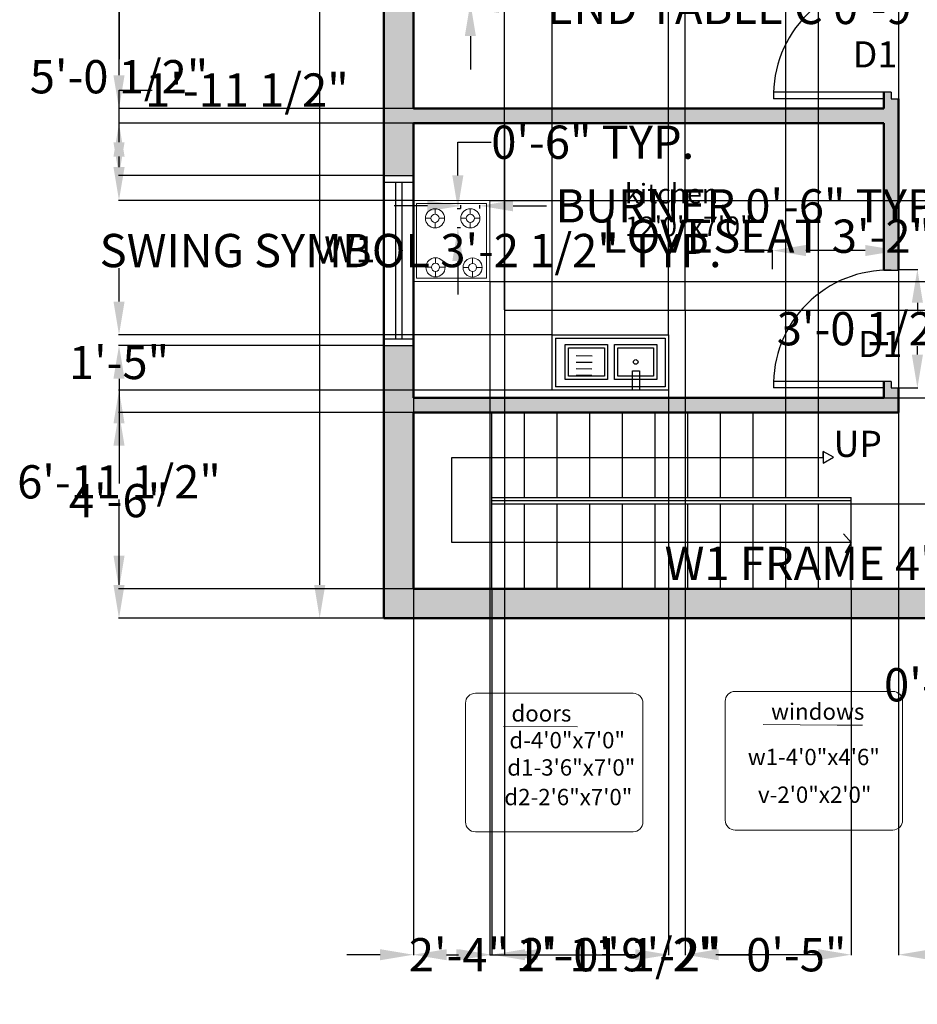
# Model space of a CAD drawing. Units: inches. Extents: x 2391 to 2964, y 130 to 798.
# Tile 1 of 4: x 2391 to 2666, y 130 to 431. Entities that reach past the tile are written whole.
import ezdxf

# ---------------------------------------------------------------- set-up
doc = ezdxf.new("R2010")
doc.units = ezdxf.units.IN
doc.header["$MEASUREMENT"] = 0
for name, color, linetype, lineweight in [('A-ANNO-DIMS', 2, 'Continuous', 18), ('A-ANNO-LEGN', 7, 'Continuous', 18), ('A-ANNO-TEXT', 7, 'Continuous', 18), ('A-AREA-IDEN', 7, 'Continuous', 25), ('A-DOOR', 3, 'Continuous', 25), ('A-EQPM', 9, 'Continuous', 18), ('A-FLOR-CASE', 8, 'Continuous', 25), ('A-FLOR-FIXT', 9, 'Continuous', 25), ('A-FLOR-STRS', 7, 'Continuous', 30), ('A-GLAZ', 4, 'Continuous', 25), ('A-WALL', 7, 'Continuous', 50)]:
    doc.layers.add(name, color=color, linetype=linetype, lineweight=lineweight)
doc.layers.add('A-WALL-PATT', color=11, linetype='Continuous', lineweight=13, true_color=0xf27172)
doc.styles.get("Standard").update_dxf_attribs({"font": 'arial.ttf'})
doc.dimstyles.get("Standard").update_dxf_attribs({"dimtxt": 10.18, "dimasz": 10.18, "dimexe": 0.18, "dimexo": 0.0625, "dimgap": 0.09, "dimtad": 0, "dimtih": 1, "dimtoh": 1, "dimdec": 0, "dimzin": 0, "dimdsep": 46, "dimlunit": 3, "dimtxsty": 'Standard', "dimcen": 0.09, "dimadec": 0, "dimazin": 0, "dimtfac": 1, "dimtdec": 0, "dimtofl": 0, "dimtmove": 0, "dimatfit": 3, "dimfxl": 1, "dimtolj": 1, "dimtzin": 0, "dimarcsym": 0})

# ---------------------------------------------------------------- blocks, each defined once
blk = doc.blocks.new('*D4')
at = {"layer": 'A-ANNO-DIMS', "color": 0, "lineweight": -2, "transparency": 16777216}
for p, q in [((2502.34, 752.24), (2482.55, 752.24)), ((2482.73, 742.06), (2482.73, 505.44)), ((2482.73, 258.42), (2482.73, 495.03)), ((2502.34, 248.24), (2482.55, 248.24))]:
    blk.add_line(p, q, dxfattribs=at)
at = {"layer": 'A-ANNO-DIMS', "color": 0, "transparency": 16777216}
for points in [[(2481.03, 742.06), (2484.43, 742.06), (2482.73, 752.24)], [(2481.03, 258.42), (2484.43, 258.42), (2482.73, 248.24)]]:
    blk.add_solid(points, dxfattribs=at)
at = {"layer": 'Defpoints', "color": 0, "transparency": 16777216}
for p in [(2502.4, 752.24), (2482.73, 248.24), (2502.4, 248.24)]:
    blk.add_point(p, dxfattribs=at)
at = {"layer": 'A-ANNO-DIMS', "color": 0, "transparency": 16777216, "insert": (2482.73, 500.24), "char_height": 10.18, "attachment_point": 5}
blk.add_mtext("\\A1;42'", dxfattribs=at)
blk = doc.blocks.new('WIN-W1-48')
for p, q in [((0, 0), (0, 9)), ((2, 0), (2, 9)), ((50, 0), (50, 9)), ((52, 0), (52, 9)), ((2, 5.5), (50, 5.5)), ((2, 3.5), (50, 3.5))]:
    blk.add_line(p, q)
blk = doc.blocks.new('DOOR-SWING-36')
for p, q in [((0, 4.5), (0, 38.25)), ((2, 2.25), (2, 38.25)), ((36, 4.5), (36, 0)), ((0, 2.25), (0, 0)), ((2, 2.25), (0, 2.25))]:
    blk.add_line(p, q)
blk.add_arc((1, 3.25), 35.01, 358.3634, 91.6366)
blk = doc.blocks.new('HOB-BURNER')
for p, q in [((2.93, 4.17), (2.93, 5.86)), ((1.69, 2.93), (0, 2.93)), ((2.93, 1.69), (2.93, 0)), ((4.17, 2.93), (5.86, 2.93))]:
    blk.add_line(p, q)
for radius in [2.93, 1.24]:
    blk.add_circle((2.93, 2.93), radius)
blk = doc.blocks.new('LEGEND-FRAME')
blk.add_line((11.62, 32.27), (34.31, 32.13))
blk.add_lwpolyline([(0, 39.41, -0.414214), (3, 42.41), (51.31, 42.41, -0.414214), (54.31, 39.41), (54.31, 3, -0.414214), (51.31, 0), (3, 0, -0.414214), (0, 3)], format="xyb", close=True)
blk = doc.blocks.new('*D15')
at = {"layer": 'A-ANNO-DIMS', "color": 0, "lineweight": -2, "transparency": 16777216}
for p, q in [((2735.63, 257.3), (2735.63, 265.22)), ((2787.63, 257.3), (2787.63, 265.22)), ((2735.63, 265.04), (2725.45, 265.04)), ((2777.45, 265.04), (2745.81, 265.04))]:
    blk.add_line(p, q, dxfattribs=at)
at = {"layer": 'A-ANNO-DIMS', "color": 0, "transparency": 16777216}
for points in [[(2745.81, 266.73), (2745.81, 263.34), (2735.63, 265.04)], [(2777.45, 266.73), (2777.45, 263.34), (2787.63, 265.04)]]:
    blk.add_solid(points, dxfattribs=at)
at = {"layer": 'Defpoints', "color": 0, "transparency": 16777216}
for p in [(2735.63, 265.04), (2735.63, 257.24), (2787.63, 257.24)]:
    blk.add_point(p, dxfattribs=at)
at = {"layer": 'A-ANNO-DIMS', "color": 0, "transparency": 16777216, "insert": (2654.62, 265.04), "char_height": 10.18, "attachment_point": 5}
blk.add_mtext('\\A1;W1 FRAME 4\'-4" TYP.', dxfattribs=at)
blk = doc.blocks.new('*D16')
at = {"layer": 'A-ANNO-DIMS', "color": 0, "lineweight": -2, "transparency": 16777216}
for p, q in [((2727.83, 267.42), (2727.83, 277.6)), ((2735.57, 257.24), (2727.65, 257.24)), ((2735.57, 248.24), (2727.65, 248.24)), ((2727.83, 238.06), (2727.83, 227.88)), ((2727.83, 227.88), (2717.65, 227.88))]:
    blk.add_line(p, q, dxfattribs=at)
at = {"layer": 'A-ANNO-DIMS', "color": 0, "transparency": 16777216}
for points in [[(2726.14, 267.42), (2729.53, 267.42), (2727.83, 257.24)], [(2726.14, 238.06), (2729.53, 238.06), (2727.83, 248.24)]]:
    blk.add_solid(points, dxfattribs=at)
at = {"layer": 'Defpoints', "color": 0, "transparency": 16777216}
for p in [(2735.63, 257.24), (2727.83, 248.24), (2735.63, 248.24)]:
    blk.add_point(p, dxfattribs=at)
at = {"layer": 'A-ANNO-DIMS', "color": 0, "transparency": 16777216, "insert": (2686.54, 227.88), "char_height": 10.18, "attachment_point": 5}
blk.add_mtext('\\A1;0\'-9" TYP.', dxfattribs=at)
blk = doc.blocks.new('*D17')
at = {"layer": 'A-ANNO-DIMS', "color": 0, "lineweight": -2, "transparency": 16777216}
for p, q in [((2621.37, 360.79), (2611.19, 360.79)), ((2621.37, 355.07), (2621.37, 360.97)), ((2649.72, 360.79), (2631.55, 360.79)), ((2659.9, 355.07), (2659.9, 360.97))]:
    blk.add_line(p, q, dxfattribs=at)
at = {"layer": 'A-ANNO-DIMS', "color": 0, "transparency": 16777216}
for points in [[(2631.55, 362.49), (2631.55, 359.09), (2621.37, 360.79)], [(2649.72, 362.49), (2649.72, 359.09), (2659.9, 360.79)]]:
    blk.add_solid(points, dxfattribs=at)
at = {"layer": 'Defpoints', "color": 0, "transparency": 16777216}
for p in [(2621.37, 360.79), (2621.37, 355.01), (2659.9, 355.01)]:
    blk.add_point(p, dxfattribs=at)
at = {"layer": 'A-ANNO-DIMS', "color": 0, "transparency": 16777216, "insert": (2510.56, 360.79), "char_height": 10.18, "attachment_point": 5}
blk.add_mtext('\\A1;SWING SYMBOL 3\'-2 1/2" TYP.', dxfattribs=at)
blk = doc.blocks.new('*D18')
at = {"layer": 'A-ANNO-DIMS', "color": 0, "lineweight": -2, "transparency": 16777216}
for p, q in [((2659.96, 355.01), (2665.86, 355.01)), ((2665.68, 344.83), (2665.68, 342.23)), ((2665.68, 328.92), (2665.68, 331.52)), ((2659.96, 318.74), (2665.86, 318.74))]:
    blk.add_line(p, q, dxfattribs=at)
at = {"layer": 'A-ANNO-DIMS', "color": 0, "transparency": 16777216}
for points in [[(2663.98, 344.83), (2667.38, 344.83), (2665.68, 355.01)], [(2663.98, 328.92), (2667.38, 328.92), (2665.68, 318.74)]]:
    blk.add_solid(points, dxfattribs=at)
at = {"layer": 'Defpoints', "color": 0, "transparency": 16777216}
for p in [(2659.9, 355.01), (2665.68, 355.01), (2659.9, 318.74)]:
    blk.add_point(p, dxfattribs=at)
at = {"layer": 'A-ANNO-DIMS', "color": 0, "transparency": 16777216, "insert": (2665.68, 336.87), "char_height": 10.18, "attachment_point": 5}
blk.add_mtext('\\A1;3\'-0 1/2" TYP.', dxfattribs=at)
blk = doc.blocks.new('*D25')
at = {"layer": 'A-ANNO-DIMS', "color": 0, "lineweight": -2, "transparency": 16777216}
for p, q in [((2507.85, 435.2), (2497.67, 435.2)), ((2518.03, 436.55), (2518.03, 435.02)), ((2527.43, 436.55), (2527.43, 435.02)), ((2537.61, 435.2), (2547.79, 435.2))]:
    blk.add_line(p, q, dxfattribs=at)
at = {"layer": 'A-ANNO-DIMS', "color": 0, "transparency": 16777216}
for points in [[(2507.85, 436.9), (2507.85, 433.5), (2518.03, 435.2)], [(2537.61, 436.9), (2537.61, 433.5), (2527.43, 435.2)]]:
    blk.add_solid(points, dxfattribs=at)
at = {"layer": 'Defpoints', "color": 0, "transparency": 16777216}
for p in [(2518.03, 436.61), (2527.43, 436.61), (2527.43, 435.2)]:
    blk.add_point(p, dxfattribs=at)
at = {"layer": 'A-ANNO-DIMS', "color": 0, "transparency": 16777216, "insert": (2639.1, 435.2), "char_height": 10.18, "attachment_point": 5}
blk.add_mtext('\\A1;END TABLE C 0\'-9 1/2" TYP.', dxfattribs=at)
blk = doc.blocks.new('*D26')
at = {"layer": 'A-ANNO-DIMS', "color": 0, "lineweight": -2, "transparency": 16777216}
for p, q in [((2528.84, 456.03), (2528.84, 466.21)), ((2528.84, 466.21), (2539.02, 466.21)), ((2527.5, 445.85), (2529.02, 445.85)), ((2527.5, 436.61), (2529.02, 436.61)), ((2528.84, 426.43), (2528.84, 416.25))]:
    blk.add_line(p, q, dxfattribs=at)
at = {"layer": 'A-ANNO-DIMS', "color": 0, "transparency": 16777216}
for points in [[(2527.15, 456.03), (2530.54, 456.03), (2528.84, 445.85)], [(2527.15, 426.43), (2530.54, 426.43), (2528.84, 436.61)]]:
    blk.add_solid(points, dxfattribs=at)
at = {"layer": 'Defpoints', "color": 0, "transparency": 16777216}
for p in [(2527.43, 445.85), (2528.84, 445.85), (2527.43, 436.61)]:
    blk.add_point(p, dxfattribs=at)
at = {"layer": 'A-ANNO-DIMS', "color": 0, "transparency": 16777216, "insert": (2570.14, 466.21), "char_height": 10.18, "attachment_point": 5}
blk.add_mtext('\\A1;0\'-9" TYP.', dxfattribs=at)
blk = doc.blocks.new('*D27')
at = {"layer": 'A-ANNO-DIMS', "color": 0, "lineweight": -2, "transparency": 16777216}
for p, q in [((2715.98, 365.18), (2705.8, 365.18)), ((2715.98, 359.56), (2715.98, 365.36)), ((2743.69, 365.18), (2726.16, 365.18)), ((2753.87, 359.56), (2753.87, 365.36))]:
    blk.add_line(p, q, dxfattribs=at)
at = {"layer": 'A-ANNO-DIMS', "color": 0, "transparency": 16777216}
for points in [[(2726.16, 366.87), (2726.16, 363.48), (2715.98, 365.18)], [(2743.69, 366.87), (2743.69, 363.48), (2753.87, 365.18)]]:
    blk.add_solid(points, dxfattribs=at)
at = {"layer": 'Defpoints', "color": 0, "transparency": 16777216}
for p in [(2715.98, 365.18), (2715.98, 359.49), (2753.87, 359.49)]:
    blk.add_point(p, dxfattribs=at)
at = {"layer": 'A-ANNO-DIMS', "color": 0, "transparency": 16777216, "insert": (2635.39, 365.18), "char_height": 10.18, "attachment_point": 5}
blk.add_mtext('\\A1;LOVESEAT 3\'-2" TYP.', dxfattribs=at)
blk = doc.blocks.new('*D29')
at = {"layer": 'A-ANNO-DIMS', "color": 0, "lineweight": -2, "transparency": 16777216}
for p, q in [((2515.72, 374.47), (2505.54, 374.47)), ((2525.9, 373.66), (2525.9, 374.65)), ((2531.76, 373.66), (2531.76, 374.65)), ((2541.94, 374.47), (2552.12, 374.47))]:
    blk.add_line(p, q, dxfattribs=at)
at = {"layer": 'A-ANNO-DIMS', "color": 0, "transparency": 16777216}
for points in [[(2515.72, 376.17), (2515.72, 372.78), (2525.9, 374.47)], [(2541.94, 376.17), (2541.94, 372.78), (2531.76, 374.47)]]:
    blk.add_solid(points, dxfattribs=at)
at = {"layer": 'Defpoints', "color": 0, "transparency": 16777216}
for p in [(2531.76, 374.47), (2525.9, 373.59), (2531.76, 373.59)]:
    blk.add_point(p, dxfattribs=at)
at = {"layer": 'A-ANNO-DIMS', "color": 0, "transparency": 16777216, "insert": (2615.01, 374.47), "char_height": 10.18, "attachment_point": 5}
blk.add_mtext('\\A1;BURNER 0\'-6" TYP.', dxfattribs=at)
blk = doc.blocks.new('*D30')
at = {"layer": 'A-ANNO-DIMS', "color": 0, "lineweight": -2, "transparency": 16777216}
for p, q in [((2525.02, 383.77), (2525.02, 393.95)), ((2525.02, 393.95), (2535.2, 393.95)), ((2525.83, 373.59), (2524.84, 373.59)), ((2525.83, 367.73), (2524.84, 367.73)), ((2525.02, 357.55), (2525.02, 347.37))]:
    blk.add_line(p, q, dxfattribs=at)
at = {"layer": 'A-ANNO-DIMS', "color": 0, "transparency": 16777216}
for points in [[(2523.32, 383.77), (2526.71, 383.77), (2525.02, 373.59)], [(2523.32, 357.55), (2526.71, 357.55), (2525.02, 367.73)]]:
    blk.add_solid(points, dxfattribs=at)
at = {"layer": 'Defpoints', "color": 0, "transparency": 16777216}
for p in [(2525.02, 373.59), (2525.9, 373.59), (2525.9, 367.73)]:
    blk.add_point(p, dxfattribs=at)
at = {"layer": 'A-ANNO-DIMS', "color": 0, "transparency": 16777216, "insert": (2566.31, 393.95), "char_height": 10.18, "attachment_point": 5}
blk.add_mtext('\\A1;0\'-6" TYP.', dxfattribs=at)
blk = doc.blocks.new('*D33')
at = {"layer": 'A-ANNO-DIMS', "color": 0, "lineweight": -2, "transparency": 16777216}
for p, q in [((2659.9, 743.17), (2659.9, 145.07)), ((2793.4, 743.17), (2793.4, 145.07)), ((2670.08, 145.25), (2697.69, 145.25)), ((2783.22, 145.25), (2755.61, 145.25))]:
    blk.add_line(p, q, dxfattribs=at)
at = {"layer": 'A-ANNO-DIMS', "color": 0, "transparency": 16777216}
for points in [[(2670.08, 146.95), (2670.08, 143.56), (2659.9, 145.25)], [(2783.22, 146.95), (2783.22, 143.56), (2793.4, 145.25)]]:
    blk.add_solid(points, dxfattribs=at)
at = {"layer": 'Defpoints', "color": 0, "transparency": 16777216}
for p in [(2659.9, 743.24), (2793.4, 743.24), (2793.4, 145.25)]:
    blk.add_point(p, dxfattribs=at)
at = {"layer": 'A-ANNO-DIMS', "color": 0, "transparency": 16777216, "insert": (2726.65, 145.25), "char_height": 10.18, "attachment_point": 5}
blk.add_mtext('\\A1;11\'-1 1/2"', dxfattribs=at)
blk = doc.blocks.new('*D34')
at = {"layer": 'A-ANNO-DIMS', "color": 0, "lineweight": -2, "transparency": 16777216}
for p, q in [((2511.34, 536.24), (2421.12, 536.24)), ((2421.3, 526.06), (2421.3, 475.52)), ((2421.3, 414.42), (2421.3, 464.95)), ((2511.34, 404.24), (2421.12, 404.24))]:
    blk.add_line(p, q, dxfattribs=at)
at = {"layer": 'A-ANNO-DIMS', "color": 0, "transparency": 16777216}
for points in [[(2419.6, 526.06), (2423, 526.06), (2421.3, 536.24)], [(2419.6, 414.42), (2423, 414.42), (2421.3, 404.24)]]:
    blk.add_solid(points, dxfattribs=at)
at = {"layer": 'Defpoints', "color": 0, "transparency": 16777216}
for p in [(2421.3, 536.24), (2511.4, 536.24), (2511.4, 404.24)]:
    blk.add_point(p, dxfattribs=at)
at = {"layer": 'A-ANNO-DIMS', "color": 0, "transparency": 16777216, "insert": (2421.3, 470.24), "char_height": 10.18, "attachment_point": 5}
blk.add_mtext('\\A1;11\'-0"', dxfattribs=at)
blk = doc.blocks.new('*D35')
at = {"layer": 'A-ANNO-DIMS', "color": 0, "lineweight": -2, "transparency": 16777216}
for p, q in [((2511.34, 311.24), (2421.12, 311.24)), ((2421.3, 301.06), (2421.3, 289.52)), ((2421.3, 267.42), (2421.3, 278.95)), ((2511.34, 257.24), (2421.12, 257.24))]:
    blk.add_line(p, q, dxfattribs=at)
at = {"layer": 'A-ANNO-DIMS', "color": 0, "transparency": 16777216}
for points in [[(2419.6, 301.06), (2423, 301.06), (2421.3, 311.24)], [(2419.6, 267.42), (2423, 267.42), (2421.3, 257.24)]]:
    blk.add_solid(points, dxfattribs=at)
at = {"layer": 'Defpoints', "color": 0, "transparency": 16777216}
for p in [(2421.3, 311.24), (2511.4, 311.24), (2511.4, 257.24)]:
    blk.add_point(p, dxfattribs=at)
at = {"layer": 'A-ANNO-DIMS', "color": 0, "transparency": 16777216, "insert": (2421.3, 284.24), "char_height": 10.18, "attachment_point": 5}
blk.add_mtext('\\A1;4\'-6"', dxfattribs=at)
blk = doc.blocks.new('*D39')
at = {"layer": 'A-ANNO-DIMS', "color": 0, "lineweight": -2, "transparency": 16777216}
for p, q in [((2502.34, 444.24), (2421.12, 444.24)), ((2421.3, 434.06), (2421.3, 419.34)), ((2421.3, 393.92), (2421.3, 408.63)), ((2502.34, 383.74), (2421.12, 383.74))]:
    blk.add_line(p, q, dxfattribs=at)
at = {"layer": 'A-ANNO-DIMS', "color": 0, "transparency": 16777216}
for points in [[(2419.6, 434.06), (2423, 434.06), (2421.3, 444.24)], [(2419.6, 393.92), (2423, 393.92), (2421.3, 383.74)]]:
    blk.add_solid(points, dxfattribs=at)
at = {"layer": 'Defpoints', "color": 0, "transparency": 16777216}
for p in [(2421.3, 444.24), (2502.4, 444.24), (2502.4, 383.74)]:
    blk.add_point(p, dxfattribs=at)
at = {"layer": 'A-ANNO-DIMS', "color": 0, "transparency": 16777216, "insert": (2421.3, 413.99), "char_height": 10.18, "attachment_point": 5}
blk.add_mtext('\\A1;5\'-0 1/2"', dxfattribs=at)
blk = doc.blocks.new('*D41')
at = {"layer": 'A-ANNO-DIMS', "color": 0, "lineweight": -2, "transparency": 16777216}
for p, q in [((2502.34, 331.74), (2421.12, 331.74)), ((2421.3, 321.56), (2421.3, 295.34)), ((2421.3, 258.42), (2421.3, 284.63)), ((2502.34, 248.24), (2421.12, 248.24))]:
    blk.add_line(p, q, dxfattribs=at)
at = {"layer": 'A-ANNO-DIMS', "color": 0, "transparency": 16777216}
for points in [[(2419.6, 321.56), (2423, 321.56), (2421.3, 331.74)], [(2419.6, 258.42), (2423, 258.42), (2421.3, 248.24)]]:
    blk.add_solid(points, dxfattribs=at)
at = {"layer": 'Defpoints', "color": 0, "transparency": 16777216}
for p in [(2421.3, 331.74), (2502.4, 331.74), (2502.4, 248.24)]:
    blk.add_point(p, dxfattribs=at)
at = {"layer": 'A-ANNO-DIMS', "color": 0, "transparency": 16777216, "insert": (2421.3, 289.99), "char_height": 10.18, "attachment_point": 5}
blk.add_mtext('\\A1;6\'-11 1/2"', dxfattribs=at)
blk = doc.blocks.new('*D47')
at = {"layer": 'A-ANNO-DIMS', "color": 0, "lineweight": -2, "transparency": 16777216}
for p, q in [((2511.4, 257.17), (2511.4, 145.07)), ((2535.4, 257.17), (2535.4, 145.07)), ((2521.58, 145.25), (2525.22, 145.25)), ((2535.4, 145.25), (2545.58, 145.25))]:
    blk.add_line(p, q, dxfattribs=at)
at = {"layer": 'A-ANNO-DIMS', "color": 0, "transparency": 16777216}
for points in [[(2521.58, 146.95), (2521.58, 143.56), (2511.4, 145.25)], [(2525.22, 146.95), (2525.22, 143.56), (2535.4, 145.25)]]:
    blk.add_solid(points, dxfattribs=at)
at = {"layer": 'Defpoints', "color": 0, "transparency": 16777216}
for p in [(2511.4, 257.24), (2535.4, 257.24), (2535.4, 145.25)]:
    blk.add_point(p, dxfattribs=at)
at = {"layer": 'A-ANNO-DIMS', "color": 0, "transparency": 16777216, "insert": (2559.29, 145.25), "char_height": 10.18, "attachment_point": 5}
blk.add_mtext('\\A1;2\'-0"', dxfattribs=at)
blk = doc.blocks.new('*D48')
at = {"layer": 'A-ANNO-DIMS', "color": 0, "lineweight": -2, "transparency": 16777216}
for p, q in [((2535.4, 257.17), (2535.4, 145.07)), ((2645.4, 257.17), (2645.4, 145.07)), ((2545.58, 145.25), (2576.78, 145.25)), ((2635.22, 145.25), (2604.02, 145.25))]:
    blk.add_line(p, q, dxfattribs=at)
at = {"layer": 'A-ANNO-DIMS', "color": 0, "transparency": 16777216}
for points in [[(2545.58, 146.95), (2545.58, 143.56), (2535.4, 145.25)], [(2635.22, 146.95), (2635.22, 143.56), (2645.4, 145.25)]]:
    blk.add_solid(points, dxfattribs=at)
at = {"layer": 'Defpoints', "color": 0, "transparency": 16777216}
for p in [(2535.4, 257.24), (2645.4, 257.24), (2645.4, 145.25)]:
    blk.add_point(p, dxfattribs=at)
at = {"layer": 'A-ANNO-DIMS', "color": 0, "transparency": 16777216, "insert": (2590.4, 145.25), "char_height": 10.18, "attachment_point": 5}
blk.add_mtext('\\A1;9\'-2"', dxfattribs=at)
blk = doc.blocks.new('*D49')
at = {"layer": 'A-ANNO-DIMS', "color": 0, "lineweight": -2, "transparency": 16777216}
for p, q in [((2529.11, 782.34), (2518.93, 782.34)), ((2539.29, 342.63), (2539.29, 782.52)), ((2594.63, 342.63), (2594.63, 782.52)), ((2604.81, 782.34), (2614.99, 782.34))]:
    blk.add_line(p, q, dxfattribs=at)
at = {"layer": 'A-ANNO-DIMS', "color": 0, "transparency": 16777216}
for points in [[(2529.11, 784.03), (2529.11, 780.64), (2539.29, 782.34)], [(2604.81, 784.03), (2604.81, 780.64), (2594.63, 782.34)]]:
    blk.add_solid(points, dxfattribs=at)
at = {"layer": 'Defpoints', "color": 0, "transparency": 16777216}
for p in [(2594.63, 782.34), (2539.29, 342.57), (2594.63, 342.57)]:
    blk.add_point(p, dxfattribs=at)
at = {"layer": 'A-ANNO-DIMS', "color": 0, "transparency": 16777216, "insert": (2566.96, 782.34), "char_height": 10.18, "attachment_point": 5}
blk.add_mtext('\\A1;4\'-7 1/2"', dxfattribs=at)
blk = doc.blocks.new('*D50')
at = {"layer": 'A-ANNO-DIMS', "color": 0, "lineweight": -2, "transparency": 16777216}
for p, q in [((2511.4, 399.67), (2511.4, 145.07)), ((2539.29, 399.67), (2539.29, 145.07)), ((2501.22, 145.25), (2491.04, 145.25)), ((2549.47, 145.25), (2559.65, 145.25))]:
    blk.add_line(p, q, dxfattribs=at)
at = {"layer": 'A-ANNO-DIMS', "color": 0, "transparency": 16777216}
for points in [[(2501.22, 146.95), (2501.22, 143.56), (2511.4, 145.25)], [(2549.47, 146.95), (2549.47, 143.56), (2539.29, 145.25)]]:
    blk.add_solid(points, dxfattribs=at)
at = {"layer": 'Defpoints', "color": 0, "transparency": 16777216}
for p in [(2511.4, 399.74), (2539.29, 399.74), (2539.29, 145.25)]:
    blk.add_point(p, dxfattribs=at)
at = {"layer": 'A-ANNO-DIMS', "color": 0, "transparency": 16777216, "insert": (2525.35, 145.25), "char_height": 10.18, "attachment_point": 5}
blk.add_mtext('\\A1;2\'-4"', dxfattribs=at)
blk = doc.blocks.new('*D51')
at = {"layer": 'A-ANNO-DIMS', "color": 0, "lineweight": -2, "transparency": 16777216}
for p, q in [((2832.5, 342.57), (2832.5, 352.75)), ((2832.5, 352.75), (2842.68, 352.75)), ((2594.69, 342.57), (2832.68, 342.57)), ((2832.5, 325.92), (2832.5, 332.39)), ((2594.69, 315.74), (2832.68, 315.74))]:
    blk.add_line(p, q, dxfattribs=at)
at = {"layer": 'A-ANNO-DIMS', "color": 0, "transparency": 16777216}
for points in [[(2830.8, 332.39), (2834.2, 332.39), (2832.5, 342.57)], [(2830.8, 325.92), (2834.2, 325.92), (2832.5, 315.74)]]:
    blk.add_solid(points, dxfattribs=at)
at = {"layer": 'Defpoints', "color": 0, "transparency": 16777216}
for p in [(2594.63, 342.57), (2832.5, 342.57), (2594.63, 315.74)]:
    blk.add_point(p, dxfattribs=at)
at = {"layer": 'A-ANNO-DIMS', "color": 0, "transparency": 16777216, "insert": (2856.39, 352.75), "char_height": 10.18, "attachment_point": 5}
blk.add_mtext('\\A1;2\'-3"', dxfattribs=at)
blk = doc.blocks.new('*D52')
at = {"layer": 'A-ANNO-DIMS', "color": 0, "lineweight": -2, "transparency": 16777216}
for p, q in [((2615.22, 782.34), (2605.04, 782.34)), ((2625.4, 311.3), (2625.4, 782.52)), ((2635.4, 311.3), (2635.4, 782.52)), ((2645.58, 782.34), (2655.76, 782.34))]:
    blk.add_line(p, q, dxfattribs=at)
at = {"layer": 'A-ANNO-DIMS', "color": 0, "transparency": 16777216}
for points in [[(2615.22, 784.03), (2615.22, 780.64), (2625.4, 782.34)], [(2645.58, 784.03), (2645.58, 780.64), (2635.4, 782.34)]]:
    blk.add_solid(points, dxfattribs=at)
at = {"layer": 'Defpoints', "color": 0, "transparency": 16777216}
for p in [(2635.4, 782.34), (2625.4, 311.24), (2635.4, 311.24)]:
    blk.add_point(p, dxfattribs=at)
at = {"layer": 'A-ANNO-DIMS', "color": 0, "transparency": 16777216, "insert": (2673.33, 782.34), "char_height": 10.18, "attachment_point": 5}
blk.add_mtext('\\A1;0\'-10"', dxfattribs=at)
blk = doc.blocks.new('*D53')
at = {"layer": 'A-ANNO-DIMS', "color": 0, "lineweight": -2, "transparency": 16777216}
for p, q in [((2832.5, 283.24), (2832.5, 293.42)), ((2832.5, 293.42), (2842.68, 293.42)), ((2645.46, 283.24), (2832.68, 283.24)), ((2832.5, 267.42), (2832.5, 273.06)), ((2645.46, 257.24), (2832.68, 257.24))]:
    blk.add_line(p, q, dxfattribs=at)
at = {"layer": 'A-ANNO-DIMS', "color": 0, "transparency": 16777216}
for points in [[(2830.8, 273.06), (2834.2, 273.06), (2832.5, 283.24)], [(2830.8, 267.42), (2834.2, 267.42), (2832.5, 257.24)]]:
    blk.add_solid(points, dxfattribs=at)
at = {"layer": 'Defpoints', "color": 0, "transparency": 16777216}
for p in [(2645.4, 283.24), (2832.5, 283.24), (2645.4, 257.24)]:
    blk.add_point(p, dxfattribs=at)
at = {"layer": 'A-ANNO-DIMS', "color": 0, "transparency": 16777216, "insert": (2856.39, 293.42), "char_height": 10.18, "attachment_point": 5}
blk.add_mtext('\\A1;2\'-2"', dxfattribs=at)
blk = doc.blocks.new('*D54')
at = {"layer": 'A-ANNO-DIMS', "color": 0, "lineweight": -2, "transparency": 16777216}
for p, q in [((2553.9, 335.07), (2553.9, 782.52)), ((2564.08, 782.34), (2579.34, 782.34)), ((2589.52, 335.07), (2589.52, 782.52)), ((2589.52, 782.34), (2599.7, 782.34))]:
    blk.add_line(p, q, dxfattribs=at)
at = {"layer": 'A-ANNO-DIMS', "color": 0, "transparency": 16777216}
for points in [[(2564.08, 784.03), (2564.08, 780.64), (2553.9, 782.34)], [(2579.34, 784.03), (2579.34, 780.64), (2589.52, 782.34)]]:
    blk.add_solid(points, dxfattribs=at)
at = {"layer": 'Defpoints', "color": 0, "transparency": 16777216}
for p in [(2589.52, 782.34), (2553.9, 335.01), (2589.52, 335.01)]:
    blk.add_point(p, dxfattribs=at)
at = {"layer": 'A-ANNO-DIMS', "color": 0, "transparency": 16777216, "insert": (2629.23, 782.34), "char_height": 10.18, "attachment_point": 5}
blk.add_mtext('\\A1;2\'-11 1/2"', dxfattribs=at)
blk = doc.blocks.new('*D55')
at = {"layer": 'A-ANNO-DIMS', "color": 0, "lineweight": -2, "transparency": 16777216}
for p, q in [((2421.3, 345.19), (2421.3, 355.37)), ((2553.83, 335.01), (2421.12, 335.01)), ((2553.83, 318.05), (2421.12, 318.05)), ((2421.3, 307.87), (2421.3, 297.69))]:
    blk.add_line(p, q, dxfattribs=at)
at = {"layer": 'A-ANNO-DIMS', "color": 0, "transparency": 16777216}
for points in [[(2419.6, 345.19), (2423, 345.19), (2421.3, 335.01)], [(2419.6, 307.87), (2423, 307.87), (2421.3, 318.05)]]:
    blk.add_solid(points, dxfattribs=at)
at = {"layer": 'Defpoints', "color": 0, "transparency": 16777216}
for p in [(2421.3, 335.01), (2553.9, 335.01), (2553.9, 318.05)]:
    blk.add_point(p, dxfattribs=at)
at = {"layer": 'A-ANNO-DIMS', "color": 0, "transparency": 16777216, "insert": (2421.3, 326.53), "char_height": 10.18, "attachment_point": 5}
blk.add_mtext('\\A1;1\'-5"', dxfattribs=at)
blk = doc.blocks.new('*D56')
at = {"layer": 'A-ANNO-DIMS', "color": 0, "lineweight": -2, "transparency": 16777216}
for p, q in [((2511.4, 351.29), (2511.4, 145.07)), ((2534.77, 351.29), (2534.77, 145.07)), ((2521.58, 145.25), (2524.59, 145.25)), ((2534.77, 145.25), (2544.95, 145.25))]:
    blk.add_line(p, q, dxfattribs=at)
at = {"layer": 'A-ANNO-DIMS', "color": 0, "transparency": 16777216}
for points in [[(2521.58, 146.95), (2521.58, 143.56), (2511.4, 145.25)], [(2524.59, 146.95), (2524.59, 143.56), (2534.77, 145.25)]]:
    blk.add_solid(points, dxfattribs=at)
at = {"layer": 'Defpoints', "color": 0, "transparency": 16777216}
for p in [(2511.4, 351.35), (2534.77, 351.35), (2534.77, 145.25)]:
    blk.add_point(p, dxfattribs=at)
at = {"layer": 'A-ANNO-DIMS', "color": 0, "transparency": 16777216, "insert": (2573.9, 145.25), "char_height": 10.18, "attachment_point": 5}
blk.add_mtext('\\A1;1\'-11 1/2"', dxfattribs=at)
blk = doc.blocks.new('*D57')
at = {"layer": 'A-ANNO-DIMS', "color": 0, "lineweight": -2, "transparency": 16777216}
for p, q in [((2832.5, 376.14), (2832.5, 386.32)), ((2832.5, 386.32), (2842.68, 386.32)), ((2534.83, 376.14), (2832.68, 376.14)), ((2832.5, 361.53), (2832.5, 365.96)), ((2534.83, 351.35), (2832.68, 351.35))]:
    blk.add_line(p, q, dxfattribs=at)
at = {"layer": 'A-ANNO-DIMS', "color": 0, "transparency": 16777216}
for points in [[(2830.8, 365.96), (2834.2, 365.96), (2832.5, 376.14)], [(2830.8, 361.53), (2834.2, 361.53), (2832.5, 351.35)]]:
    blk.add_solid(points, dxfattribs=at)
at = {"layer": 'Defpoints', "color": 0, "transparency": 16777216}
for p in [(2534.77, 376.14), (2832.5, 376.14), (2534.77, 351.35)]:
    blk.add_point(p, dxfattribs=at)
at = {"layer": 'A-ANNO-DIMS', "color": 0, "transparency": 16777216, "insert": (2856.39, 386.32), "char_height": 10.18, "attachment_point": 5}
blk.add_mtext('\\A1;2\'-1"', dxfattribs=at)
blk = doc.blocks.new('*D58')
at = {"layer": 'A-ANNO-DIMS', "color": 0, "lineweight": -2, "transparency": 16777216}
for p, q in [((2421.3, 399.74), (2421.3, 409.92)), ((2421.3, 409.92), (2431.48, 409.92)), ((2511.34, 399.74), (2421.12, 399.74)), ((2421.3, 386.32), (2421.3, 389.56)), ((2511.34, 376.14), (2421.12, 376.14))]:
    blk.add_line(p, q, dxfattribs=at)
at = {"layer": 'A-ANNO-DIMS', "color": 0, "transparency": 16777216}
for points in [[(2419.6, 389.56), (2423, 389.56), (2421.3, 399.74)], [(2419.6, 386.32), (2423, 386.32), (2421.3, 376.14)]]:
    blk.add_solid(points, dxfattribs=at)
at = {"layer": 'Defpoints', "color": 0, "transparency": 16777216}
for p in [(2421.3, 399.74), (2511.4, 399.74), (2511.4, 376.14)]:
    blk.add_point(p, dxfattribs=at)
at = {"layer": 'A-ANNO-DIMS', "color": 0, "transparency": 16777216, "insert": (2460.44, 409.92), "char_height": 10.18, "attachment_point": 5}
blk.add_mtext('\\A1;1\'-11 1/2"', dxfattribs=at)
blk = doc.blocks.new('*D59')
at = {"layer": 'A-ANNO-DIMS', "color": 0, "lineweight": -2, "transparency": 16777216}
for p, q in [((2589.52, 317.99), (2589.52, 145.07)), ((2594.63, 315.67), (2594.63, 145.07)), ((2579.34, 145.25), (2569.16, 145.25)), ((2604.81, 145.25), (2614.99, 145.25))]:
    blk.add_line(p, q, dxfattribs=at)
at = {"layer": 'A-ANNO-DIMS', "color": 0, "transparency": 16777216}
for points in [[(2579.34, 146.95), (2579.34, 143.56), (2589.52, 145.25)], [(2604.81, 146.95), (2604.81, 143.56), (2594.63, 145.25)]]:
    blk.add_solid(points, dxfattribs=at)
at = {"layer": 'Defpoints', "color": 0, "transparency": 16777216}
for p in [(2589.52, 318.05), (2594.63, 315.74), (2594.63, 145.25)]:
    blk.add_point(p, dxfattribs=at)
at = {"layer": 'A-ANNO-DIMS', "color": 0, "transparency": 16777216, "insert": (2628.61, 145.25), "char_height": 10.18, "attachment_point": 5}
blk.add_mtext('\\A1;0\'-5"', dxfattribs=at)

msp = doc.modelspace()

# ---------------------------------------------------------------- hatches: boundary and pattern name
at = {"layer": 'A-WALL-PATT'}
h = msp.add_hatch(color=256, dxfattribs=at)
h.dxf.hatch_style = 1
h.paths.add_polyline_path([(2557.4, 752.24), (2502.4, 752.24), (2502.4, 579.74), (2511.4, 579.74), (2511.4, 594.74), (2595.4, 594.74), (2599.9, 594.74), (2616.4, 594.74), (2616.4, 596.99, -0.014283), (2616.4, 598.99), (2616.4, 599.24), (2511.4, 599.24), (2511.4, 743.24), (2557.4, 743.24)])
h.paths.add_polyline_path([(2700.65, 752.24), (2609.4, 752.24), (2609.4, 743.24), (2655.4, 743.24), (2655.4, 599.24), (2650.4, 599.24), (2650.4, 596.99), (2652.4, 596.99), (2652.4, 594.74), (2662.9, 594.74), (2662.9, 596.99), (2664.9, 596.99), (2664.9, 599.24), (2659.9, 599.24), (2659.9, 743.24), (2700.65, 743.24)])
h.paths.add_polyline_path([(2802.4, 752.24), (2752.65, 752.24), (2752.65, 743.24), (2793.4, 743.24), (2793.4, 599.24), (2698.9, 599.24), (2698.9, 598.99, -0.014283), (2698.9, 596.99), (2698.9, 594.74), (2704.9, 594.74), (2704.9, 536.24), (2737.79, 536.24), (2737.79, 540.74), (2709.4, 540.74), (2709.4, 594.74), (2793.4, 594.74), (2793.4, 581.74), (2802.4, 581.74)])
h.paths.add_polyline_path([(2511.4, 444.24), (2502.4, 444.24), (2502.4, 383.74), (2511.4, 383.74), (2511.4, 399.74), (2655.4, 399.74), (2655.4, 354.74), (2655.65, 354.74, -0.014283), (2657.65, 354.74), (2659.9, 354.74), (2659.9, 407.24), (2657.65, 407.24), (2657.65, 409.24), (2655.4, 409.24), (2655.4, 404.24), (2511.4, 404.24)])
h.paths.add_polyline_path([(2511.4, 536.24), (2599.9, 536.24), (2655.4, 536.24), (2655.4, 443.24), (2655.65, 443.24, -0.014283), (2657.65, 443.24), (2659.9, 443.24), (2659.9, 540.74), (2599.9, 540.74), (2599.9, 555.74), (2597.65, 555.74, -0.014283), (2595.65, 555.74), (2595.4, 555.74), (2595.4, 540.74), (2511.4, 540.74), (2511.4, 555.74), (2502.4, 555.74), (2502.4, 496.24), (2511.4, 496.24), (2511.4, 503.82)])
h.paths.add_polyline_path([(2676.45, 257.24), (2511.4, 257.24), (2511.4, 311.24), (2659.9, 311.24), (2659.9, 318.74), (2657.65, 318.74), (2657.65, 320.74), (2655.4, 320.74), (2655.4, 315.74), (2511.4, 315.74), (2511.4, 331.74), (2502.4, 331.74), (2502.4, 248.24), (2676.45, 248.24)])
h.paths.add_polyline_path([(2802.4, 370.74), (2793.4, 370.74), (2793.4, 257.24), (2787.63, 257.24), (2787.63, 248.24), (2802.4, 248.24)])
h.paths.add_polyline_path([(2735.63, 257.24), (2715.45, 257.24), (2715.45, 254.74, -0.014283), (2715.45, 252.74), (2715.45, 248.24), (2721.55, 248.24), (2735.63, 248.24)])
h.paths.add_polyline_path([(2802.4, 553.74), (2793.4, 553.74), (2793.4, 540.74), (2763.73, 540.74), (2763.73, 536.24), (2793.4, 536.24), (2793.4, 422.74), (2802.4, 422.74)])

# ---------------------------------------------------------------- linework, layer by layer
at = {"layer": 'A-ANNO-LEGN'}
msp.add_line((2641.17, 215.54), (2648.91, 215.49), dxfattribs=at)
at = {"layer": 'A-EQPM'}
for points in [[(2534.77, 376.14), (2511.4, 376.14), (2511.4, 351.35), (2534.77, 351.35)], [(2533.77, 375.14), (2512.4, 375.14), (2512.4, 352.35), (2533.77, 352.35)]]:
    msp.add_lwpolyline(points, close=True, dxfattribs=at)
at = {"layer": 'A-FLOR-CASE'}
for p, q in [((2539.29, 399.74), (2539.29, 342.57)), ((2539.29, 342.57), (2594.63, 342.57)), ((2594.63, 342.57), (2594.63, 315.74))]:
    msp.add_line(p, q, dxfattribs=at)
at = {"layer": 'A-FLOR-FIXT'}
for p, q in [((2554.9, 334.01), (2554.9, 319.05)), ((2561.26, 328.66), (2566.1, 328.61)), ((2561.24, 326.66), (2566.08, 326.61)), ((2561.19, 322.66), (2566.04, 322.61)), ((2561.22, 324.66), (2566.06, 324.61))]:
    msp.add_line(p, q, dxfattribs=at)
for points in [[(2553.9, 318.05), (2553.9, 335.01), (2589.52, 335.01), (2589.52, 318.05)], [(2557.87, 332.05), (2570.86, 332.05), (2570.86, 321.3), (2557.87, 321.3)], [(2572.96, 332.05), (2585.95, 332.05), (2585.95, 321.3), (2572.96, 321.3)], [(2558.87, 331.05), (2569.86, 331.05), (2569.86, 322.3), (2558.87, 322.3)], [(2573.96, 331.05), (2584.95, 331.05), (2584.95, 322.3), (2573.96, 322.3)], [(2580.61, 318.05), (2578.48, 318.05), (2578.48, 323.99), (2580.61, 323.99)]]:
    msp.add_lwpolyline(points, close=True, dxfattribs=at)
msp.add_lwpolyline([(2554.9, 334.01), (2588.52, 334.01), (2588.52, 319.05), (2554.9, 319.05)], dxfattribs=at)
msp.add_circle((2579.46, 326.68), 0.709, dxfattribs=at)
at = {"layer": 'A-FLOR-STRS'}
for p, q in [((2535.4, 257.24), (2535.4, 311.24)), ((2545.4, 285.24), (2545.4, 311.24)), ((2555.4, 285.24), (2555.4, 311.24)), ((2565.4, 285.24), (2565.4, 311.24)), ((2575.4, 285.24), (2575.4, 311.24)), ((2585.4, 285.24), (2585.4, 311.24)), ((2595.4, 285.24), (2595.4, 311.24)), ((2605.4, 285.24), (2605.4, 311.24)), ((2615.4, 285.24), (2615.4, 311.24)), ((2625.4, 285.24), (2625.4, 311.24)), ((2635.4, 285.24), (2635.4, 311.24)), ((2636.84, 297.49), (2636.84, 299.29)), ((2636.84, 299.29), (2636.84, 295.74)), ((2640.04, 297.59), (2636.84, 299.29)), ((2523.13, 271.47), (2523.13, 297.49)), ((2523.13, 297.49), (2636.84, 297.49)), ((2636.84, 295.74), (2640.04, 297.59)), ((2535.4, 285.24), (2645.4, 285.24)), ((2535.4, 284.24), (2645.4, 284.24)), ((2645.4, 257.24), (2645.4, 285.24)), ((2535.4, 283.24), (2645.4, 283.24)), ((2545.4, 257.24), (2545.4, 283.24)), ((2555.4, 257.24), (2555.4, 283.24)), ((2565.4, 257.24), (2565.4, 283.24)), ((2575.4, 257.24), (2575.4, 283.24)), ((2585.4, 257.24), (2585.4, 283.24)), ((2595.4, 257.24), (2595.4, 283.24)), ((2605.4, 257.24), (2605.4, 283.24)), ((2615.4, 257.24), (2615.4, 283.24)), ((2625.4, 257.24), (2625.4, 283.24)), ((2635.4, 257.24), (2635.4, 283.24)), ((2645.4, 271.47), (2523.13, 271.47)), ((2645.4, 271.47), (2643.11, 274.12)), ((2643.11, 274.12), (2645.4, 271.47)), ((2645.4, 271.47), (2643.55, 268.27))]:
    msp.add_line(p, q, dxfattribs=at)
at = {"layer": 'A-GLAZ'}
msp.add_line((2507.9, 381.74), (2507.9, 333.74), dxfattribs=at)
at = {"layer": 'A-WALL'}
for p, q in [((2502.4, 248.24), (2502.4, 752.24)), ((2511.4, 404.24), (2511.4, 536.24)), ((2655.4, 404.24), (2655.4, 409.24)), ((2655.4, 404.24), (2655.4, 409.24)), ((2659.9, 399.74), (2659.9, 407.24)), ((2659.9, 354.74), (2659.9, 407.24)), ((2511.4, 404.24), (2655.4, 404.24)), ((2511.4, 399.74), (2655.4, 399.74)), ((2511.4, 315.74), (2511.4, 399.74)), ((2655.4, 354.73), (2655.4, 399.74)), ((2655.4, 315.74), (2655.4, 320.74)), ((2659.9, 311.24), (2659.9, 318.74)), ((2511.4, 315.74), (2655.4, 315.74)), ((2511.4, 257.24), (2511.4, 311.24)), ((2511.4, 311.24), (2659.9, 311.24)), ((2681.45, 257.24), (2511.4, 257.24)), ((2679.45, 248.24), (2502.4, 248.24))]:
    msp.add_line(p, q, dxfattribs=at)

# ---------------------------------------------------------------- block references
at = {"layer": 'A-ANNO-LEGN'}
for p in [(2527.37, 182.87), (2606.86, 183.42)]:
    msp.add_blockref('LEGEND-FRAME', p, dxfattribs=at)
at = {"layer": 'A-DOOR'}
for p, rotation in [((2659.9, 407.24), 89.99999999999888), ((2659.9, 318.74), 89.9999999999989)]:
    msp.add_blockref('DOOR-SWING-36', p, dxfattribs=dict(at, rotation=rotation))
at = {"layer": 'A-EQPM'}
for p in [(2515.1, 367.73), (2525.9, 367.73), (2515.25, 352.72), (2526.6, 352.67)]:
    msp.add_blockref('HOB-BURNER', p, dxfattribs=at)
at = {"layer": 'A-GLAZ', "rotation": 269.999999999996}
msp.add_blockref('WIN-W1-48', (2502.4, 383.73), dxfattribs=at)

# ---------------------------------------------------------------- texts
at = {"layer": 'A-ANNO-TEXT', "attachment_point": 1}
for s, width, insert, char_height in [('D1', 35.9617, (2645.92, 424.83), 8), ('W1', 35.9617, (2484.11, 365.17), 8), ('D1', 35.9617, (2647.48, 336.18), 8), ('UP', 35.9617, (2640.04, 305.62), 8), ('doors', 20.8895, (2541.42, 221.62), 5), ('windows', 20.8895, (2620.9, 222.17), 5), ('d-4\'0"x7\'0"', 20.8895, (2540.79, 213.42), 5), ('w1-4\'0"x4\'6"', 20.8895, (2613.77, 208.27), 5), ('d1-3\'6"x7\'0"', 20.8895, (2540.15, 205.07), 5), ('d2-2\'6"x7\'0"', 20.8895, (2539.24, 196.01), 5), ('v-2\'0"x2\'0"', 20.8895, (2616.89, 196.73), 5)]:
    msp.add_mtext_dynamic_manual_height_columns(s, width=width, gutter_width=1, heights=[0], dxfattribs=dict(at, insert=insert, char_height=char_height))
at = {"layer": 'A-AREA-IDEN', "insert": (2576.18, 381.21), "char_height": 6, "attachment_point": 1}
msp.add_mtext_dynamic_manual_height_columns('kitchen\\P12\'0"x7\'0"', width=87.7895, gutter_width=1, heights=[0], dxfattribs=at)

# ---------------------------------------------------------------- dimensions: what is measured, and where the dimension line sits
at = {"layer": 'A-ANNO-DIMS'}
for base, p1, p2, picture, middle in [((2594.63, 782.34), (2539.29, 342.57), (2594.63, 342.57), '*D49', (2566.96, 782.34)), ((2589.52, 782.34), (2553.9, 335.01), (2589.52, 335.01), '*D54', (2629.23, 782.34)), ((2635.4, 782.34), (2625.4, 311.24), (2635.4, 311.24), '*D52', (2673.33, 782.34)), ((2793.4, 145.25), (2659.9, 743.24), (2793.4, 743.24), '*D33', (2726.65, 145.25)), ((2539.29, 145.25), (2511.4, 399.74), (2539.29, 399.74), '*D50', (2525.35, 145.25)), ((2534.77, 145.25), (2511.4, 351.35), (2534.77, 351.35), '*D56', (2573.9, 145.25)), ((2594.63, 145.25), (2589.52, 318.05), (2594.63, 315.74), '*D59', (2628.61, 145.25)), ((2535.4, 145.25), (2511.4, 257.24), (2535.4, 257.24), '*D47', (2559.29, 145.25)), ((2645.4, 145.25), (2535.4, 257.24), (2645.4, 257.24), '*D48', (2590.4, 145.25))]:
    dim = msp.add_linear_dim(base=base, p1=p1, p2=p2, dimstyle='Standard', override={"dimdec": 1, "dimlfac": 1, "dimrnd": 0, "dimzin": 1, "dimdsep": 46, "dimlunit": 4, "dimfrac": 2}, dxfattribs=at)
    dim.commit()
    dim.dimension.update_dxf_attribs({"geometry": picture, "text_midpoint": middle})
for base, p1, p2, override, picture, middle in [((2482.73, 248.24), (2502.4, 752.24), (2502.4, 248.24), {"dimclrd": 0, "dimclre": 0, "dimclrt": 0}, '*D4', (2482.73, 500.24)), ((2421.3, 536.24), (2511.4, 404.24), (2511.4, 536.24), {"dimdec": 1, "dimlfac": 1, "dimrnd": 0, "dimzin": 1, "dimdsep": 46, "dimlunit": 4, "dimfrac": 2}, '*D34', (2421.3, 470.24)), ((2421.3, 444.24), (2502.4, 383.74), (2502.4, 444.24), {"dimdec": 1, "dimlfac": 1, "dimrnd": 0, "dimzin": 1, "dimdsep": 46, "dimlunit": 4, "dimfrac": 2}, '*D39', (2421.3, 413.99)), ((2421.3, 399.74), (2511.4, 376.14), (2511.4, 399.74), {"dimdec": 1, "dimlfac": 1, "dimrnd": 0, "dimzin": 1, "dimdsep": 46, "dimlunit": 4, "dimfrac": 2}, '*D58', (2460.44, 409.92)), ((2832.5, 376.14), (2534.77, 351.35), (2534.77, 376.14), {"dimdec": 1, "dimlfac": 1, "dimrnd": 0, "dimzin": 1, "dimdsep": 46, "dimlunit": 4, "dimfrac": 2}, '*D57', (2856.39, 386.32)), ((2832.5, 342.57), (2594.63, 315.74), (2594.63, 342.57), {"dimdec": 1, "dimlfac": 1, "dimrnd": 0, "dimzin": 1, "dimdsep": 46, "dimlunit": 4, "dimfrac": 2}, '*D51', (2856.39, 352.75)), ((2421.3, 335.01), (2553.9, 318.05), (2553.9, 335.01), {"dimdec": 1, "dimlfac": 1, "dimrnd": 0, "dimzin": 1, "dimdsep": 46, "dimlunit": 4, "dimfrac": 2}, '*D55', (2421.3, 326.53)), ((2421.3, 331.74), (2502.4, 248.24), (2502.4, 331.74), {"dimdec": 1, "dimlfac": 1, "dimrnd": 0, "dimzin": 1, "dimdsep": 46, "dimlunit": 4, "dimfrac": 2}, '*D41', (2421.3, 289.99)), ((2421.3, 311.24), (2511.4, 257.24), (2511.4, 311.24), {"dimdec": 1, "dimlfac": 1, "dimrnd": 0, "dimzin": 1, "dimdsep": 46, "dimlunit": 4, "dimfrac": 2}, '*D35', (2421.3, 284.24)), ((2832.5, 283.24), (2645.4, 257.24), (2645.4, 283.24), {"dimdec": 1, "dimlfac": 1, "dimrnd": 0, "dimzin": 1, "dimdsep": 46, "dimlunit": 4, "dimfrac": 2}, '*D53', (2856.39, 293.42))]:
    dim = msp.add_linear_dim(base=base, p1=p1, p2=p2, angle=90, dimstyle='Standard', override=override, dxfattribs=at)
    dim.commit()
    dim.dimension.update_dxf_attribs({"geometry": picture, "text_midpoint": middle})
for base, p1, p2, text, picture, middle in [((2527.43, 435.2), (2518.03, 436.61), (2527.43, 436.61), 'END TABLE C <> TYP.', '*D25', (2639.1, 435.2)), ((2531.76, 374.47), (2525.9, 373.59), (2531.76, 373.59), 'BURNER <> TYP.', '*D29', (2615.01, 374.47))]:
    dim = msp.add_linear_dim(base=base, p1=p1, p2=p2, text=text, dimstyle='Standard', override={"dimdec": 1, "dimlfac": 1, "dimrnd": 0, "dimzin": 1, "dimdsep": 46, "dimlunit": 4, "dimfrac": 2}, dxfattribs=at)
    dim.commit()
    dim.dimension.update_dxf_attribs({"geometry": picture, "text_midpoint": middle})
for base, p1, p2, angle, text, picture, middle in [((2528.84, 445.85), (2527.43, 436.61), (2527.43, 445.85), 90, '<> TYP.', '*D26', (2570.14, 466.21)), ((2525.02, 373.59), (2525.9, 367.73), (2525.9, 373.59), 90, '<> TYP.', '*D30', (2566.31, 393.95)), ((2621.37, 360.79), (2659.9, 355.01), (2621.37, 355.01), 180, 'SWING SYMBOL <> TYP.', '*D17', (2510.56, 360.79)), ((2715.98, 365.18), (2753.87, 359.49), (2715.98, 359.49), 180, 'LOVESEAT <> TYP.', '*D27', (2635.39, 365.18)), ((2665.68, 355.01), (2659.9, 318.74), (2659.9, 355.01), 90, '<> TYP.', '*D18', (2665.68, 336.87)), ((2735.63, 265.04), (2787.63, 257.24), (2735.63, 257.24), 180, 'W1 FRAME <> TYP.', '*D15', (2654.62, 265.04)), ((2727.83, 248.24), (2735.63, 257.24), (2735.63, 248.24), 270, '<> TYP.', '*D16', (2686.54, 227.88))]:
    dim = msp.add_linear_dim(base=base, p1=p1, p2=p2, angle=angle, text=text, dimstyle='Standard', override={"dimdec": 1, "dimlfac": 1, "dimrnd": 0, "dimzin": 1, "dimdsep": 46, "dimlunit": 4, "dimfrac": 2}, dxfattribs=at)
    dim.commit()
    dim.dimension.update_dxf_attribs({"geometry": picture, "text_midpoint": middle})

doc.saveas('drawing.dxf')
